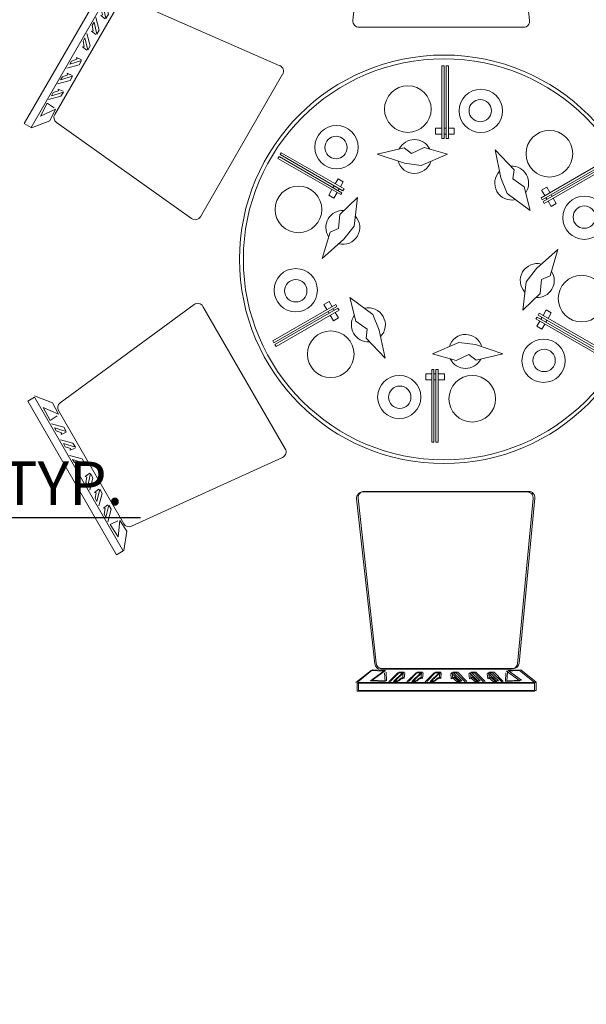
# Model space of a CAD drawing. Units: inches. Extents: x 1239 to 2276906, y 2273 to 321338.
# Tile 3 of 23: x 1424 to 1482, y 2408 to 2510. Entities that reach past the tile are written whole.
import ezdxf

# ---------------------------------------------------------------- set-up
doc = ezdxf.new("R2010")
doc.units = ezdxf.units.IN
doc.layers.add('A-ANNO-DIMS', color=2, linetype='Continuous', lineweight=18)
doc.layers.add('A-FURN', color=8, linetype='Continuous', lineweight=13)
doc.styles.get("Standard").update_dxf_attribs({"font": 'arial.ttf'})
doc.dimstyles.new('ISO-25', dxfattribs={"dimtxt": 4.5, "dimasz": 4, "dimexe": 1.25, "dimexo": 0.625, "dimtad": 1, "dimdec": 1, "dimlunit": 3, "dimtxsty": 'Standard', "dimcen": 2.5, "dimadec": 0, "dimazin": 0, "dimtfac": 1, "dimtdec": 1, "dimtmove": 0, "dimatfit": 3, "dimfxl": 1, "dimarcsym": 0})

# ---------------------------------------------------------------- blocks, each defined once
blk = doc.blocks.new('A$C45501D90')
for p, q in [((-242.2, 1133.5), (224, 1133.5)), ((-242.2, 1112.8), (-242.2, 1133.5)), ((224, 1133.5), (224, 1112.8)), ((224, 1112.8), (-242.2, 1112.8)), ((-242.2, 1111.2), (-202.3, 1079.2)), ((-203.9, 1106.4), (-165.6, 1108)), ((-168.8, 1080.8), (-203.9, 1106.4)), ((-165.6, 1108), (-167.2, 1085.6)), ((-156, 1109.6), (-132, 1085.6)), ((-119.3, 1085.6), (-143.2, 1108)), ((-143.2, 1108), (-133.6, 1108)), ((-133.6, 1108), (-122.5, 1098.4)), ((-122.5, 1098.4), (-119.3, 1101.6)), ((-119.3, 1101.6), (-117.7, 1087.2)), ((-108.1, 1109.6), (-84.1, 1085.6)), ((-71.4, 1085.6), (-95.3, 1108)), ((-95.3, 1108), (-85.7, 1108)), ((-85.7, 1108), (-74.6, 1098.4)), ((-74.6, 1098.4), (-71.4, 1101.6)), ((-71.4, 1101.6), (-69.8, 1087.2)), ((-60.2, 1109.6), (-36.2, 1085.6)), ((-23.5, 1085.6), (-47.4, 1108)), ((-47.4, 1108), (-37.8, 1108)), ((-37.8, 1108), (-26.7, 1098.4)), ((-26.7, 1098.4), (-23.5, 1101.6)), ((-23.5, 1101.6), (-21.9, 1087.2)), ((8.5, 1101.6), (6.9, 1087.2)), ((8.5, 1085.6), (32.4, 1108)), ((11.6, 1098.4), (8.5, 1101.6)), ((22.8, 1108), (11.6, 1098.4)), ((45.2, 1109.6), (21.2, 1085.6)), ((32.4, 1108), (22.8, 1108)), ((56.3, 1101.6), (54.8, 1087.2)), ((56.3, 1085.6), (80.3, 1108)), ((59.5, 1098.4), (56.3, 1101.6)), ((70.7, 1108), (59.5, 1098.4)), ((93.1, 1109.6), (69.1, 1085.6)), ((80.3, 1108), (70.7, 1108)), ((104.2, 1101.6), (102.6, 1087.2)), ((104.2, 1085.6), (128.2, 1108)), ((107.4, 1098.4), (104.2, 1101.6)), ((118.6, 1108), (107.4, 1098.4)), ((141, 1109.6), (117, 1085.6)), ((128.2, 1108), (118.6, 1108)), ((188.9, 1106.4), (150.5, 1108)), ((150.5, 1108), (152.1, 1085.6)), ((153.7, 1080.8), (188.9, 1106.4)), ((224, 1112.8), (187.3, 1079.2)), ((-197.3, 1061.6), (-238.9, 627.6)), ((-202.3, 1079.2), (-168.8, 1080.8)), ((161.8, 1076.1), (-181.4, 1076.1)), ((-132, 1085.6), (-119.3, 1085.6)), ((-84.1, 1085.6), (-71.4, 1085.6)), ((-36.2, 1085.6), (-23.5, 1085.6)), ((21.2, 1085.6), (8.5, 1085.6)), ((69.1, 1085.6), (56.3, 1085.6)), ((117, 1085.6), (104.2, 1085.6)), ((187.3, 1079.2), (153.7, 1080.8)), ((225.2, 627.8), (177.6, 1061.8)), ((842.6, 766.1), (860.5, 776.5)), ((860.5, 776.5), (1093.6, 372.8)), ((-1102.7, 357), (-869.7, 760.7)), ((-869.7, 760.7), (-851.7, 750.4)), ((-848.7, 752.3), (-841, 701.8)), ((841.2, 765.3), (833.5, 714.8)), ((1075.7, 362.4), (842.6, 766.1)), ((-851.7, 750.4), (-1084.8, 346.6)), ((851.7, 686.6), (856.2, 729.8)), ((856.2, 729.8), (876.7, 697.4)), ((-863.7, 716.7), (-884.3, 684.4)), ((-859.2, 673.6), (-863.7, 716.7)), ((-841, 701.8), (-859.2, 673.6)), ((820.7, 701.7), (424.1, 520.7)), ((833.5, 714.8), (851.7, 686.6)), ((-851, 678.1), (-1022.6, 380.9)), ((-890.4, 676.9), (-881.7, 644.2)), ((-884.3, 684.4), (-864.1, 674.6)), ((-431.1, 509), (-830.8, 684.8)), ((1012.8, 397.9), (841.2, 695.1)), ((876.7, 697.4), (856.6, 687.6)), ((882.9, 689.9), (874.2, 657.2)), ((880.6, 646.1), (887.9, 678)), ((887.9, 678), (892.7, 669.7)), ((-895.4, 665), (-900.2, 656.7)), ((-900.2, 656.7), (-897.5, 642.2)), ((-888.1, 633.1), (-895.4, 665)), ((874.2, 657.2), (880.6, 646.1)), ((894.4, 654.1), (882.7, 645.5)), ((892.7, 669.7), (890, 655.2)), ((890, 655.2), (894.4, 654.1)), ((906.9, 648.4), (898.1, 615.7)), ((-919.4, 623.5), (-924.2, 615.2)), ((-912, 591.6), (-919.4, 623.5)), ((-914.4, 635.4), (-905.6, 602.7)), ((-897.5, 642.2), (-901.9, 641.1)), ((-901.9, 641.1), (-890.2, 632.5)), ((-881.7, 644.2), (-888.1, 633.1)), ((904.5, 604.6), (911.9, 636.5)), ((911.9, 636.5), (916.7, 628.2)), ((916.7, 628.2), (914, 613.8)), ((-921.5, 600.8), (-925.8, 599.6)), ((-925.8, 599.6), (-914.2, 591)), ((-924.2, 615.2), (-921.5, 600.8)), ((-905.6, 602.7), (-912, 591.6)), ((-223, 610.1), (209.4, 610.1)), ((898.1, 615.7), (904.5, 604.6)), ((918.3, 612.6), (906.7, 604)), ((914, 613.8), (918.3, 612.6)), ((930.8, 606.9), (922.1, 574.2)), ((-943.3, 582), (-948.1, 573.8)), ((-948.1, 573.8), (-945.4, 559.3)), ((-936, 550.1), (-943.3, 582)), ((-938.3, 593.9), (-929.6, 561.2)), ((922.1, 574.2), (928.4, 563.1)), ((928.4, 563.1), (935.8, 595.1)), ((942.3, 571.1), (930.6, 562.6)), ((935.8, 595.1), (940.6, 586.8)), ((940.6, 586.8), (937.9, 572.3)), ((937.9, 572.3), (942.3, 571.1)), ((-945.4, 559.3), (-949.8, 558.1)), ((-949.8, 558.1), (-938.1, 549.6)), ((-929.6, 561.2), (-936, 550.1)), ((-951.9, 522.5), (-983.2, 512.9)), ((-983.2, 512.9), (-978.5, 521.2)), ((-978.5, 521.2), (-964.6, 526.1)), ((-964.6, 526.1), (-965.7, 530.5)), ((-965.7, 530.5), (-952.5, 524.7)), ((-958.3, 511.4), (-951.9, 522.5)), ((950.8, 524.4), (944.4, 535.5)), ((944.4, 535.5), (975.7, 525.9)), ((958.2, 543.5), (945, 537.7)), ((983.5, 515.7), (950.8, 524.4)), ((957.1, 539.1), (958.2, 543.5)), ((970.9, 534.2), (957.1, 539.1)), ((975.7, 525.9), (970.9, 534.2)), ((-991, 502.7), (-958.3, 511.4)), ((-5.6, 508.7, 90.8), (0.4, 508.7, 90.8)), ((-5.6, 317.7, 90.8), (-5.6, 508.7, 90.8)), ((0.4, 508.7, 90.8), (0.4, 317.7, 90.8)), ((5.8, 317.7, 90.8), (5.8, 508.7, 90.8)), ((5.8, 508.7, 90.8), (11.8, 508.7, 90.8)), ((11.8, 508.7, 90.8), (11.8, 317.7, 90.8)), ((416.9, 498.2), (633.1, 123.7)), ((968.4, 494), (999.7, 484.4)), ((974.7, 483), (968.4, 494)), ((982.2, 502), (968.9, 496.2)), ((981, 497.6), (982.2, 502)), ((994.9, 492.7), (981, 497.6)), ((999.7, 484.4), (994.9, 492.7)), ((-1015, 461.2), (-982.3, 469.9)), ((-975.9, 481), (-1007.2, 471.4)), ((-1007.2, 471.4), (-1002.4, 479.7)), ((-1002.4, 479.7), (-988.5, 484.6)), ((-988.5, 484.6), (-989.7, 489)), ((-989.7, 489), (-976.5, 483.2)), ((-982.3, 469.9), (-975.9, 481)), ((-639.9, 111.9), (-423.7, 486.4)), ((1007.4, 474.2), (974.7, 483)), ((-1026.3, 438.3), (-1012.5, 443.1)), ((-1012.5, 443.1), (-1013.6, 447.5)), ((-1013.6, 447.5), (-1000.4, 441.7)), ((998.7, 441.5), (992.3, 452.5)), ((992.3, 452.5), (1023.6, 443)), ((1006.1, 460.5), (992.9, 454.7)), ((1031.4, 432.7), (998.7, 441.5)), ((1005, 456.2), (1006.1, 460.5)), ((1018.8, 451.3), (1005, 456.2)), ((1023.6, 443), (1018.8, 451.3)), ((-1038.9, 419.7), (-1006.2, 428.5)), ((-999.8, 439.5), (-1031.1, 430)), ((-1031.1, 430), (-1026.3, 438.3)), ((-1006.2, 428.5), (-999.8, 439.5)), ((1034.8, 423.6), (1016.3, 411.1)), ((1052.6, 389.6), (1034.8, 423.6)), ((-1060.1, 376.6), (-1042.3, 410.6)), ((-1020.4, 394.3), (-1060.1, 376.6)), ((-1042.3, 410.6), (-1023.8, 398.1)), ((-1035.8, 364.4), (-1020.4, 394.3)), ((1028.3, 377.5), (1012.9, 407.3)), ((1012.9, 407.3), (1052.6, 389.6)), ((-1083.4, 345.8), (-1035.8, 364.4)), ((656.3, 118.9), (1008.4, 377.1)), ((1075.9, 358.8), (1028.3, 377.5)), ((1093.6, 372.8), (1075.7, 362.4)), ((-1084.8, 346.6), (-1102.7, 357)), ((-1018, 360), (-663, 106.9)), ((-22.3, 329.1, 90.8), (-22.3, 344.6, 90.8)), ((-22.3, 344.6, 90.8), (-5.6, 344.6, 90.8)), ((0.4, 344.6, 90.8), (5.8, 344.6, 90.8)), ((11.8, 344.6, 90.8), (27.3, 344.6, 90.8)), ((27.3, 344.6, 90.8), (27.3, 329.1, 90.8)), ((-5.6, 329.1, 90.8), (-22.3, 329.1, 90.8)), ((0.4, 317.7, 90.8), (-5.6, 317.7, 90.8)), ((5.8, 329.1, 90.8), (0.4, 329.1, 90.8)), ((11.8, 317.7, 90.8), (5.8, 317.7, 90.8)), ((27.3, 329.1, 90.8), (11.8, 329.1, 90.8)), ((-175.3, 276.1, 90.8), (-104.8, 293.2, 90.8)), ((-104.8, 293.2, 90.8), (-85.5, 278.4, 90.8)), ((-85.5, 278.4, 90.8), (-52.1, 293.9, 90.8)), ((-52.1, 293.9, 90.8), (9.5, 276.1, 90.8)), ((134.3, 288, 90.8), (184.3, 235.5, 90.8)), ((149.7, 213.9, 90.8), (134.3, 288, 90.8)), ((-436.3, 265.3, 90.8), (-433.3, 270.5, 90.8)), ((-270.9, 169.9, 90.8), (-436.3, 265.3, 90.8)), ((-433.3, 270.5, 90.8), (-267.9, 175, 90.8)), ((-430.6, 275.2, 90.8), (-427.6, 280.3, 90.8)), ((-265.2, 179.7, 90.8), (-430.6, 275.2, 90.8)), ((-427.6, 280.3, 90.8), (-262.3, 184.9, 90.8)), ((-103.3, 252.4, 90.8), (-175.3, 276.1, 90.8)), ((9.5, 276.1, 90.8), (-59.5, 246.5, 90.8)), ((-59.5, 246.5, 90.8), (-103.3, 252.4, 90.8)), ((184.3, 235.5, 90.8), (181.1, 211.4, 90.8)), ((255.2, 161.9, 90.8), (420.6, 257.3, 90.8)), ((423.5, 252.2, 90.8), (258.2, 156.7, 90.8)), ((260.9, 152, 90.8), (426.2, 247.5, 90.8)), ((429.2, 242.3, 90.8), (263.8, 146.9, 90.8)), ((420.6, 257.3, 90.8), (423.5, 252.2, 90.8)), ((426.2, 247.5, 90.8), (429.2, 242.3, 90.8)), ((-285.5, 198.3, 90.8), (-277.8, 211.7, 90.8)), ((-277.8, 211.7, 90.8), (-264.3, 204, 90.8)), ((166.5, 173, 90.8), (149.7, 213.9, 90.8)), ((181.1, 211.4, 90.8), (211.3, 190.3, 90.8)), ((-302.5, 168.8, 90.8), (-294.2, 183.3, 90.8)), ((-291.2, 188.5, 90.8), (-288.5, 193.1, 90.8)), ((-275.1, 185.4, 90.8), (-277.8, 180.7, 90.8)), ((-264.3, 204, 90.8), (-272.1, 190.5, 90.8)), ((-262.3, 184.9, 90.8), (-265.2, 179.7, 90.8)), ((211.3, 190.3, 90.8), (226.7, 128.1, 90.8)), ((256.6, 182, 90.8), (270.1, 189.8, 90.8)), ((265, 167.5, 90.8), (256.6, 182, 90.8)), ((270.1, 189.8, 90.8), (278.4, 175.3, 90.8)), ((-289.1, 161.1, 90.8), (-302.5, 168.8, 90.8)), ((-280.7, 175.5, 90.8), (-289.1, 161.1, 90.8)), ((-273.6, 117.6, 90.8), (-227.4, 162.1, 90.8)), ((-267.9, 175, 90.8), (-270.9, 169.9, 90.8)), ((-227.4, 162.1, 90.8), (-236.2, 87.5, 90.8)), ((226.7, 128.1, 90.8), (166.5, 173, 90.8)), ((258.2, 156.7, 90.8), (255.2, 161.9, 90.8)), ((270.7, 157.7, 90.8), (268, 162.4, 90.8)), ((281.4, 170.1, 90.8), (284.1, 165.5, 90.8)), ((287.1, 160.3, 90.8), (294.9, 146.8, 90.8)), ((263.8, 146.9, 90.8), (260.9, 152, 90.8)), ((281.4, 139.1, 90.8), (273.7, 152.5, 90.8)), ((294.9, 146.8, 90.8), (281.4, 139.1, 90.8)), ((-276.8, 80.9, 90.8), (-273.6, 117.6, 90.8)), ((-299.3, 71.7, 90.8), (-276.8, 80.9, 90.8)), ((-236.2, 87.5, 90.8), (-263.2, 52.5, 90.8)), ((-319.8, 2.1, 90.8), (-299.3, 71.7, 90.8)), ((-263.2, 52.5, 90.8), (-319.8, 2.1, 90.8)), ((242.9, -24.6, 90.8), (299.4, 25.9, 90.8)), ((299.4, 25.9, 90.8), (278.9, -43.7, 90.8)), ((215.8, -59.5, 90.8), (242.9, -24.6, 90.8)), ((278.9, -43.7, 90.8), (256.4, -53, 90.8)), ((207, -134.1, 90.8), (215.8, -59.5, 90.8)), ((256.4, -53, 90.8), (253.2, -89.7, 90.8)), ((-247, -100.1, 90.8), (-186.8, -145, 90.8)), ((-231.7, -162.3, 90.8), (-247, -100.1, 90.8)), ((253.2, -89.7, 90.8), (207, -134.1, 90.8)), ((-656.3, -118.9), (-1008.4, -377.1)), ((-416.9, -498.2), (-633.1, -123.7)), ((-449.6, -214.4, 90.8), (-284.2, -118.9, 90.8)), ((-281.2, -124.1, 90.8), (-446.6, -219.5, 90.8)), ((-443.9, -224.2, 90.8), (-278.5, -128.7, 90.8)), ((-315.2, -118.9, 90.8), (-301.8, -111.1, 90.8)), ((-307.5, -132.3, 90.8), (-315.2, -118.9, 90.8)), ((-301.8, -111.1, 90.8), (-294, -124.6, 90.8)), ((-284.2, -118.9, 90.8), (-281.2, -124.1, 90.8)), ((-278.5, -128.7, 90.8), (-275.5, -133.9, 90.8)), ((639.9, -111.9), (423.7, -486.4)), ((1018, -360), (663, -106.9)), ((-275.5, -133.9, 90.8), (-440.9, -229.4, 90.8)), ((-301.8, -142.1, 90.8), (-304.5, -137.5, 90.8)), ((-290.4, -161.8, 90.8), (-298.8, -147.3, 90.8)), ((-291, -129.7, 90.8), (-288.3, -134.4, 90.8)), ((-277, -154, 90.8), (-290.4, -161.8, 90.8)), ((-285.4, -139.5, 90.8), (-277, -154, 90.8)), ((-186.8, -145, 90.8), (-170.1, -185.9, 90.8)), ((241.9, -156.9, 90.8), (244.9, -151.7, 90.8)), ((244.9, -151.7, 90.8), (410.3, -247.2, 90.8)), ((247.6, -147.1, 90.8), (250.6, -141.9, 90.8)), ((413, -242.5, 90.8), (247.6, -147.1, 90.8)), ((250.6, -141.9, 90.8), (415.9, -237.4, 90.8)), ((254.7, -157.4, 90.8), (257.4, -152.7, 90.8)), ((260.4, -147.6, 90.8), (268.7, -133.1, 90.8)), ((268.7, -133.1, 90.8), (282.2, -140.8, 90.8)), ((282.2, -140.8, 90.8), (273.8, -155.3, 90.8)), ((-201.5, -183.4, 90.8), (-231.7, -162.3, 90.8)), ((407.3, -252.4, 90.8), (241.9, -156.9, 90.8)), ((244, -176, 90.8), (251.7, -162.5, 90.8)), ((257.4, -183.7, 90.8), (244, -176, 90.8)), ((265.2, -170.3, 90.8), (257.4, -183.7, 90.8)), ((270.8, -160.5, 90.8), (268.1, -165.1, 90.8)), ((-204.7, -207.6, 90.8), (-201.5, -183.4, 90.8)), ((-170.1, -185.9, 90.8), (-154.7, -260.1, 90.8)), ((-446.6, -219.5, 90.8), (-449.6, -214.4, 90.8)), ((-440.9, -229.4, 90.8), (-443.9, -224.2, 90.8)), ((-154.7, -260.1, 90.8), (-204.7, -207.6, 90.8)), ((-29.8, -248.2, 90.8), (39.2, -218.5, 90.8)), ((39.2, -218.5, 90.8), (83, -224.4, 90.8)), ((83, -224.4, 90.8), (154.9, -248.2, 90.8)), ((31.8, -266, 90.8), (-29.8, -248.2, 90.8)), ((65.2, -250.4, 90.8), (31.8, -266, 90.8)), ((84.4, -265.2, 90.8), (65.2, -250.4, 90.8)), ((154.9, -248.2, 90.8), (84.4, -265.2, 90.8)), ((410.3, -247.2, 90.8), (407.3, -252.4, 90.8)), ((415.9, -237.4, 90.8), (413, -242.5, 90.8)), ((-47.6, -316.6, 90.8), (-47.6, -301.1, 90.8)), ((-47.6, -301.1, 90.8), (-32.1, -301.1, 90.8)), ((-32.1, -480.7, 90.8), (-32.1, -289.8, 90.8)), ((-32.1, -289.8, 90.8), (-26.1, -289.8, 90.8)), ((-26.1, -289.8, 90.8), (-26.1, -480.7, 90.8)), ((-26.1, -301.1, 90.8), (-20.8, -301.1, 90.8)), ((-20.8, -480.7, 90.8), (-20.8, -289.8, 90.8)), ((-20.8, -289.8, 90.8), (-14.8, -289.8, 90.8)), ((-14.8, -289.8, 90.8), (-14.8, -480.7, 90.8)), ((-14.8, -301.1, 90.8), (1.9, -301.1, 90.8)), ((1.9, -301.1, 90.8), (1.9, -316.6, 90.8)), ((-32.1, -316.6, 90.8), (-47.6, -316.6, 90.8)), ((-20.8, -316.6, 90.8), (-26.1, -316.6, 90.8)), ((1.9, -316.6, 90.8), (-14.8, -316.6, 90.8)), ((-1075.9, -358.8), (-1028.3, -377.5)), ((851.7, -750.4), (1084.8, -346.6)), ((1102.7, -357), (869.7, -760.7)), ((1083.4, -345.8), (1035.8, -364.4)), ((1084.8, -346.6), (1102.7, -357)), ((-1093.6, -372.8), (-1075.7, -362.4)), ((-860.5, -776.5), (-1093.6, -372.8)), ((-1075.7, -362.4), (-842.6, -766.1)), ((-1028.3, -377.5), (-1012.9, -407.3)), ((851, -678.1), (1022.6, -380.9)), ((1035.8, -364.4), (1020.4, -394.3)), ((1020.4, -394.3), (1060.1, -376.6)), ((1060.1, -376.6), (1042.3, -410.6)), ((-1052.6, -389.6), (-1034.8, -423.6)), ((-1012.9, -407.3), (-1052.6, -389.6)), ((-1034.8, -423.6), (-1016.3, -411.1)), ((-1012.8, -397.9), (-841.2, -695.1)), ((1042.3, -410.6), (1023.8, -398.1)), ((-1031.4, -432.7), (-998.7, -441.5)), ((1006.2, -428.5), (999.8, -439.5)), ((999.8, -439.5), (1031.1, -430)), ((1038.9, -419.7), (1006.2, -428.5)), ((1026.3, -438.3), (1012.5, -443.1)), ((1031.1, -430), (1026.3, -438.3)), ((-1023.6, -443), (-1018.8, -451.3)), ((-992.3, -452.5), (-1023.6, -443)), ((-1018.8, -451.3), (-1005, -456.2)), ((-1006.1, -460.5), (-992.9, -454.7)), ((-1005, -456.2), (-1006.1, -460.5)), ((-998.7, -441.5), (-992.3, -452.5)), ((1015, -461.2), (982.3, -469.9)), ((1013.6, -447.5), (1000.4, -441.7)), ((1012.5, -443.1), (1013.6, -447.5)), ((-1007.4, -474.2), (-974.7, -483)), ((-968.4, -494), (-999.7, -484.4)), ((-999.7, -484.4), (-994.9, -492.7)), ((-974.7, -483), (-968.4, -494)), ((-26.1, -480.7, 90.8), (-32.1, -480.7, 90.8)), ((-14.8, -480.7, 90.8), (-20.8, -480.7, 90.8)), ((982.3, -469.9), (975.9, -481)), ((975.9, -481), (1007.2, -471.4)), ((989.7, -489), (976.5, -483.2)), ((1002.4, -479.7), (988.5, -484.6)), ((988.5, -484.6), (989.7, -489)), ((1007.2, -471.4), (1002.4, -479.7)), ((-994.9, -492.7), (-981, -497.6)), ((-983.5, -515.7), (-950.8, -524.4)), ((-982.2, -502), (-968.9, -496.2)), ((-981, -497.6), (-982.2, -502)), ((431.1, -509), (830.8, -684.8)), ((958.3, -511.4), (951.9, -522.5)), ((951.9, -522.5), (983.2, -512.9)), ((991, -502.7), (958.3, -511.4)), ((983.2, -512.9), (978.5, -521.2)), ((-944.4, -535.5), (-975.7, -525.9)), ((-975.7, -525.9), (-970.9, -534.2)), ((-970.9, -534.2), (-957.1, -539.1)), ((-958.2, -543.5), (-945, -537.7)), ((-957.1, -539.1), (-958.2, -543.5)), ((-950.8, -524.4), (-944.4, -535.5)), ((-820.7, -701.7), (-424.1, -520.7)), ((965.7, -530.5), (952.5, -524.7)), ((978.5, -521.2), (964.6, -526.1)), ((964.6, -526.1), (965.7, -530.5)), ((-942.3, -571.1), (-930.6, -562.6)), ((-928.4, -563.1), (-935.8, -595.1)), ((-922.1, -574.2), (-928.4, -563.1)), ((929.6, -561.2), (936, -550.1)), ((938.3, -593.9), (929.6, -561.2)), ((936, -550.1), (943.3, -582)), ((949.8, -558.1), (938.1, -549.6)), ((945.4, -559.3), (949.8, -558.1)), ((948.1, -573.8), (945.4, -559.3)), ((-937.9, -572.3), (-942.3, -571.1)), ((-940.6, -586.8), (-937.9, -572.3)), ((-935.8, -595.1), (-940.6, -586.8)), ((-930.8, -606.9), (-922.1, -574.2)), ((905.6, -602.7), (912, -591.6)), ((912, -591.6), (919.4, -623.5)), ((925.8, -599.6), (914.2, -591)), ((943.3, -582), (948.1, -573.8)), ((-918.3, -612.6), (-906.7, -604)), ((-914, -613.8), (-918.3, -612.6)), ((-916.7, -628.2), (-914, -613.8)), ((-904.5, -604.6), (-911.9, -636.5)), ((-906.9, -648.4), (-898.1, -615.7)), ((-898.1, -615.7), (-904.5, -604.6)), ((218.9, -611.6), (-213.5, -611.6)), ((223, -610.1), (-209.4, -610.1)), ((914.4, -635.4), (905.6, -602.7)), ((919.4, -623.5), (924.2, -615.2)), ((921.5, -600.8), (925.8, -599.6)), ((924.2, -615.2), (921.5, -600.8)), ((-911.9, -636.5), (-916.7, -628.2)), ((-894.4, -654.1), (-882.7, -645.5)), ((-880.6, -646.1), (-887.9, -678)), ((-874.2, -657.2), (-880.6, -646.1)), ((-229.3, -629.3), (-181.8, -1063.3)), ((-225.2, -627.8), (-177.6, -1061.8)), ((193.2, -1063.1), (234.8, -629.1)), ((197.3, -1061.6), (238.9, -627.6)), ((881.7, -644.2), (888.1, -633.1)), ((890.4, -676.9), (881.7, -644.2)), ((888.1, -633.1), (895.4, -665)), ((901.9, -641.1), (890.2, -632.5)), ((897.5, -642.2), (901.9, -641.1)), ((900.2, -656.7), (897.5, -642.2)), ((-890, -655.2), (-894.4, -654.1)), ((-892.7, -669.7), (-890, -655.2)), ((-887.9, -678), (-892.7, -669.7)), ((-882.9, -689.9), (-874.2, -657.2)), ((895.4, -665), (900.2, -656.7)), ((-876.7, -697.4), (-856.6, -687.6)), ((-856.2, -729.8), (-876.7, -697.4)), ((-851.7, -686.6), (-856.2, -729.8)), ((-833.5, -714.8), (-851.7, -686.6)), ((841, -701.8), (859.2, -673.6)), ((859.2, -673.6), (863.7, -716.7)), ((863.7, -716.7), (884.3, -684.4)), ((884.3, -684.4), (864.1, -674.6)), ((-841.2, -765.3), (-833.5, -714.8)), ((848.7, -752.3), (841, -701.8)), ((869.7, -760.7), (851.7, -750.4)), ((-842.6, -766.1), (-860.5, -776.5)), ((-231.3, -1112.7), (-191.4, -1080.8)), ((-227.2, -1111.2), (-187.3, -1079.2)), ((-157.9, -1082.4), (-193, -1107.9)), ((-191.4, -1080.8), (-157.9, -1082.4)), ((-153.7, -1080.8), (-188.9, -1106.4)), ((-187.3, -1079.2), (-153.7, -1080.8)), ((-165.9, -1077.6), (177.3, -1077.6)), ((-161.8, -1076.1), (181.4, -1076.1)), ((-150.5, -1108), (-152.1, -1085.6)), ((-141, -1109.6), (-117, -1085.6)), ((-104.2, -1085.6), (-128.2, -1108)), ((-117, -1085.6), (-104.2, -1085.6)), ((-93.1, -1109.6), (-69.1, -1085.6)), ((-56.3, -1085.6), (-80.3, -1108)), ((-69.1, -1085.6), (-56.3, -1085.6)), ((-45.2, -1109.6), (-21.2, -1085.6)), ((-8.5, -1085.6), (-32.4, -1108)), ((-21.2, -1085.6), (-8.5, -1085.6)), ((23.5, -1085.6), (47.4, -1108)), ((36.2, -1085.6), (23.5, -1085.6)), ((60.2, -1109.6), (36.2, -1085.6)), ((71.4, -1085.6), (95.3, -1108)), ((84.1, -1085.6), (71.4, -1085.6)), ((108.1, -1109.6), (84.1, -1085.6)), ((119.3, -1085.6), (143.2, -1108)), ((132, -1085.6), (119.3, -1085.6)), ((156, -1109.6), (132, -1085.6)), ((198.2, -1080.8), (164.6, -1082.4)), ((164.6, -1082.4), (199.8, -1107.9)), ((165.6, -1108), (167.2, -1085.6)), ((202.3, -1079.2), (168.8, -1080.8)), ((168.8, -1080.8), (203.9, -1106.4)), ((238.1, -1112.7), (198.2, -1080.8)), ((242.2, -1111.2), (202.3, -1079.2)), ((-224, -1112.8), (242.2, -1112.8)), ((-224, -1133.5), (-224, -1112.8)), ((-193, -1107.9), (-154.7, -1109.5)), ((-188.9, -1106.4), (-150.5, -1108)), ((-154.7, -1109.5), (-156.3, -1087.1)), ((-145.1, -1111.1), (-121.1, -1087.1)), ((-108.4, -1087.1), (-132.3, -1109.5)), ((-132.3, -1109.5), (-122.7, -1109.5)), ((-128.2, -1108), (-118.6, -1108)), ((-122.7, -1109.5), (-111.6, -1099.9)), ((-121.1, -1087.1), (-108.4, -1087.1)), ((-118.6, -1108), (-107.4, -1098.4)), ((-111.6, -1099.9), (-108.4, -1103.1)), ((-108.4, -1103.1), (-106.8, -1088.7)), ((-107.4, -1098.4), (-104.2, -1101.6)), ((-104.2, -1101.6), (-102.6, -1087.2)), ((-97.2, -1111.1), (-73.2, -1087.1)), ((-60.5, -1087.1), (-84.4, -1109.5)), ((-84.4, -1109.5), (-74.8, -1109.5)), ((-80.3, -1108), (-70.7, -1108)), ((-74.8, -1109.5), (-63.7, -1099.9)), ((-73.2, -1087.1), (-60.5, -1087.1)), ((-70.7, -1108), (-59.5, -1098.4)), ((-63.7, -1099.9), (-60.5, -1103.1)), ((-60.5, -1103.1), (-58.9, -1088.7)), ((-59.5, -1098.4), (-56.3, -1101.6)), ((-56.3, -1101.6), (-54.8, -1087.2)), ((-49.3, -1111.1), (-25.3, -1087.1)), ((-12.6, -1087.1), (-36.5, -1109.5)), ((-36.5, -1109.5), (-26.9, -1109.5)), ((-32.4, -1108), (-22.8, -1108)), ((-26.9, -1109.5), (-15.8, -1099.9)), ((-25.3, -1087.1), (-12.6, -1087.1)), ((-22.8, -1108), (-11.6, -1098.4)), ((-15.8, -1099.9), (-12.6, -1103.1)), ((-12.6, -1103.1), (-11, -1088.7)), ((-11.6, -1098.4), (-8.5, -1101.6)), ((-8.5, -1101.6), (-6.9, -1087.2)), ((19.4, -1103.1), (17.8, -1088.7)), ((19.4, -1087.1), (43.3, -1109.5)), ((32.1, -1087.1), (19.4, -1087.1)), ((22.6, -1099.9), (19.4, -1103.1)), ((23.5, -1101.6), (21.9, -1087.2)), ((33.7, -1109.5), (22.6, -1099.9)), ((26.7, -1098.4), (23.5, -1101.6)), ((37.8, -1108), (26.7, -1098.4)), ((56.1, -1111.1), (32.1, -1087.1)), ((43.3, -1109.5), (33.7, -1109.5)), ((47.4, -1108), (37.8, -1108)), ((67.3, -1103.1), (65.7, -1088.7)), ((67.3, -1087.1), (91.2, -1109.5)), ((80, -1087.1), (67.3, -1087.1)), ((70.4, -1099.9), (67.3, -1103.1)), ((71.4, -1101.6), (69.8, -1087.2)), ((81.6, -1109.5), (70.4, -1099.9)), ((74.6, -1098.4), (71.4, -1101.6)), ((85.7, -1108), (74.6, -1098.4)), ((104, -1111.1), (80, -1087.1)), ((91.2, -1109.5), (81.6, -1109.5)), ((95.3, -1108), (85.7, -1108)), ((115.1, -1103.1), (113.6, -1088.7)), ((115.1, -1087.1), (139.1, -1109.5)), ((127.9, -1087.1), (115.1, -1087.1)), ((118.3, -1099.9), (115.1, -1103.1)), ((119.3, -1101.6), (117.7, -1087.2)), ((129.5, -1109.5), (118.3, -1099.9)), ((122.5, -1098.4), (119.3, -1101.6)), ((133.6, -1108), (122.5, -1098.4)), ((151.9, -1111.1), (127.9, -1087.1)), ((139.1, -1109.5), (129.5, -1109.5)), ((143.2, -1108), (133.6, -1108)), ((161.4, -1109.5), (163, -1087.1)), ((199.8, -1107.9), (161.4, -1109.5)), ((203.9, -1106.4), (165.6, -1108)), ((242.2, -1112.8), (242.2, -1133.5)), ((-228.1, -1114.3), (238.1, -1114.3)), ((-228.1, -1135), (-228.1, -1114.3)), ((238.1, -1135), (-228.1, -1135)), ((242.2, -1133.5), (-224, -1133.5)), ((238.1, -1114.3), (238.1, -1135))]:
    blk.add_line(p, q)
for centre, radius in [((0, 0), 537), ((0, 0), 527), ((-94.8, 394.7, 90.8), 61.3), ((96.9, 390, 90.8), 56.9), ((95.5, 390.7, 90.8), 29.4), ((-282.3, 294.7, 90.8), 56.9), ((277.2, 277.6, 90.8), 61.3), ((-283.5, 293.9, 90.8), 29.4), ((-382.1, 131.1, 90.8), 61.3), ((369, 109.3, 90.8), 56.9), ((368.9, 110.8, 90.8), 29.4), ((-389.3, -81.3, 90.8), 56.9), ((361.8, -103.1, 90.8), 61.3), ((-389.2, -82.8, 90.8), 29.4), ((-297.5, -249.6, 90.8), 61.3), ((261.9, -266.7, 90.8), 56.9), ((263.2, -265.9, 90.8), 29.4), ((-117.2, -362, 90.8), 56.9), ((74.4, -366.7, 90.8), 61.3), ((-115.9, -362.7, 90.8), 29.4)]:
    blk.add_circle(centre, radius)
for centre, radius, start, end in [((-181.4, 1060.1), 16, 90, 174.5199), ((161.8, 1060.1), 16, 6.2572, 90), ((827.4, 687.1), 16, 30, 114.5199), ((-837.2, 670.1), 16, 66.2572, 150), ((-223, 626.1), 16, 174.5199, 270), ((209.4, 626.1), 16, 270, 6.2572), ((430.7, 506.2), 16, 114.5199, 210), ((-437.5, 494.4), 16, 330, 66.2572), ((999, 389.9), 16, 306.2572, 30), ((-1008.8, 373), 16, 150, 234.5199), ((-77.3, 270.2, 90.8), 44.6, 25.8558, 153.3359), ((-77.3, 270.2, 90.8), 44.6, 195.9338, 342.9389), ((178.1, 200.3, 90.8), 44.6, 325.8558, 93.3359), ((178.1, 200.3, 90.8), 44.6, 135.9338, 282.9389), ((-653.7, 119.9), 16, 234.5199, 330), ((-265.7, 83.9, 90.8), 44.6, 85.8558, 213.3359), ((-265.7, 83.9, 90.8), 44.6, 255.9338, 42.9389), ((646.9, 131.7), 16, 210, 306.2572), ((245.3, -55.9, 90.8), 44.6, 75.9338, 222.9389), ((245.3, -55.9, 90.8), 44.6, 265.8558, 33.3359), ((-646.9, -131.7), 16, 30, 126.2572), ((-198.5, -172.3, 90.8), 44.6, 315.9338, 102.9389), ((653.7, -119.9), 16, 54.5199, 150), ((-198.5, -172.3, 90.8), 44.6, 145.8558, 273.3359), ((57, -242.2, 90.8), 44.6, 15.9338, 162.9389), ((57, -242.2, 90.8), 44.6, 205.8558, 333.3359), ((1008.8, -373), 16, 330, 54.5199), ((-999, -389.9), 16, 126.2572, 210), ((437.5, -494.4), 16, 150, 246.2572), ((-430.7, -506.2), 16, 294.5199, 30), ((-213.5, -627.6), 16, 90, 186.2572), ((-209.4, -626.1), 16, 90, 186.2572), ((218.9, -627.6), 16, 354.5199, 90), ((223, -626.1), 16, 354.5199, 90), ((-827.4, -687.1), 16, 210, 294.5199), ((837.2, -670.1), 16, 246.2572, 330), ((-165.9, -1061.6), 16, 186.2572, 270), ((-161.8, -1060.1), 16, 186.2572, 270), ((177.3, -1061.6), 16, 270, 354.5199), ((181.4, -1060.1), 16, 270, 354.5199)]:
    blk.add_arc(centre, radius, start, end)
blk = doc.blocks.new('*D78')
at = {"layer": 'A-ANNO-DIMS', "color": 0, "lineweight": -2, "transparency": 16777216}
for p, q in [((1340.71, 2454.19), (1340.71, 2459.76)), ((1373.67, 2454.19), (1373.67, 2459.76)), ((1344.71, 2458.51), (1369.67, 2458.51)), ((1373.67, 2458.51), (1436.02, 2458.51))]:
    blk.add_line(p, q, dxfattribs=at)
at = {"layer": 'A-ANNO-DIMS', "color": 0, "transparency": 16777216}
for points in [[(1344.71, 2459.18), (1344.71, 2457.84), (1340.71, 2458.51)], [(1369.67, 2459.18), (1369.67, 2457.84), (1373.67, 2458.51)]]:
    blk.add_solid(points, dxfattribs=at)
at = {"layer": 'Defpoints', "color": 0, "transparency": 16777216}
for p in [(1373.67, 2458.51), (1340.71, 2453.57), (1373.67, 2453.57)]:
    blk.add_point(p, dxfattribs=at)
at = {"layer": 'A-ANNO-DIMS', "color": 0, "transparency": 16777216, "insert": (1406.85, 2461.46), "char_height": 4.5, "attachment_point": 5}
blk.add_mtext('SHRUB B 2\'-9" TYP.', dxfattribs=at)
blk = doc.blocks.new('*D89')
at = {"layer": 'A-ANNO-DIMS', "color": 0, "lineweight": -2, "transparency": 16777216}
for p, q in [((1359.38, 3215.77), (1359.38, 2275.7)), ((1551.38, 3215.77), (1551.38, 2275.7)), ((1363.38, 2276.95), (1547.38, 2276.95))]:
    blk.add_line(p, q, dxfattribs=at)
at = {"layer": 'A-ANNO-DIMS', "color": 0, "transparency": 16777216}
for points in [[(1363.38, 2277.61), (1363.38, 2276.28), (1359.38, 2276.95)], [(1547.38, 2277.61), (1547.38, 2276.28), (1551.38, 2276.95)]]:
    blk.add_solid(points, dxfattribs=at)
at = {"layer": 'Defpoints', "color": 0, "transparency": 16777216}
for p in [(1359.38, 3216.4), (1551.38, 3216.4), (1551.38, 2276.95)]:
    blk.add_point(p, dxfattribs=at)
at = {"layer": 'A-ANNO-DIMS', "color": 0, "transparency": 16777216, "insert": (1455.38, 2279.87), "char_height": 4.5, "attachment_point": 5}
blk.add_mtext('16\'-0"', dxfattribs=at)
blk = doc.blocks.new('*D103')
at = {"layer": 'A-ANNO-DIMS', "color": 0, "lineweight": -2, "transparency": 16777216}
for p, q in [((1539.93, 2607.52), (1247.33, 2607.52)), ((1248.58, 2353.9), (1248.58, 2603.52)), ((1539.93, 2349.9), (1247.33, 2349.9))]:
    blk.add_line(p, q, dxfattribs=at)
at = {"layer": 'A-ANNO-DIMS', "color": 0, "transparency": 16777216}
for points in [[(1247.92, 2603.52), (1249.25, 2603.52), (1248.58, 2607.52)], [(1247.92, 2353.9), (1249.25, 2353.9), (1248.58, 2349.9)]]:
    blk.add_solid(points, dxfattribs=at)
at = {"layer": 'Defpoints', "color": 0, "transparency": 16777216}
for p in [(1248.58, 2607.52), (1540.55, 2607.52), (1540.55, 2349.9)]:
    blk.add_point(p, dxfattribs=at)
at = {"layer": 'A-ANNO-DIMS', "color": 0, "transparency": 16777216, "insert": (1245.63, 2478.71), "char_height": 4.5, "attachment_point": 5, "rotation": 90}
blk.add_mtext('21\'-5 1/2"', dxfattribs=at)

msp = doc.modelspace()

# ---------------------------------------------------------------- block references
at = {"layer": 'A-FURN', "xscale": 0.0393700787401575, "yscale": 0.0393700787401575, "zscale": 0.0393700787401575}
msp.add_blockref('A$C45501D90', (1467.4, 2485.22), dxfattribs=at)

# ---------------------------------------------------------------- dimensions: what is measured, and where the dimension line sits
at = {"layer": 'A-ANNO-DIMS'}
dim = msp.add_linear_dim(base=(1551.38, 2276.95), p1=(1359.38, 3216.4), p2=(1551.38, 3216.4), dimstyle='ISO-25', override={"dimdec": 1, "dimlfac": 1, "dimrnd": 0, "dimzin": 1, "dimdsep": 46, "dimlunit": 4, "dimfrac": 2}, dxfattribs=at)
dim.commit()
dim.dimension.update_dxf_attribs({"geometry": '*D89', "text_midpoint": (1455.38, 2279.87)})
dim = msp.add_linear_dim(base=(1248.58, 2607.52), p1=(1540.55, 2349.9), p2=(1540.55, 2607.52), angle=90, dimstyle='ISO-25', override={"dimdec": 1, "dimlfac": 1, "dimrnd": 0, "dimzin": 1, "dimdsep": 46, "dimlunit": 4, "dimfrac": 2}, dxfattribs=at)
dim.commit()
dim.dimension.update_dxf_attribs({"geometry": '*D103', "text_midpoint": (1245.63, 2478.71)})
dim = msp.add_linear_dim(base=(1373.67, 2458.51), p1=(1340.71, 2453.57), p2=(1373.67, 2453.57), text='SHRUB B <> TYP.', dimstyle='ISO-25', override={"dimdec": 1, "dimlfac": 1, "dimrnd": 0, "dimzin": 1, "dimdsep": 46, "dimlunit": 4, "dimfrac": 2}, dxfattribs=at)
dim.commit()
dim.dimension.update_dxf_attribs({"geometry": '*D78', "text_midpoint": (1406.85, 2461.46)})

doc.saveas('drawing.dxf')
